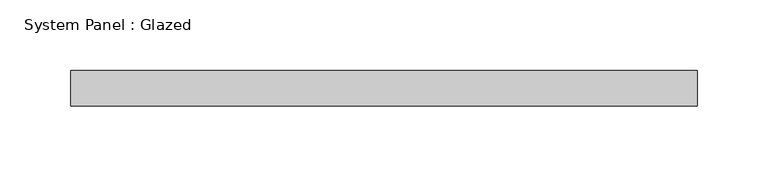
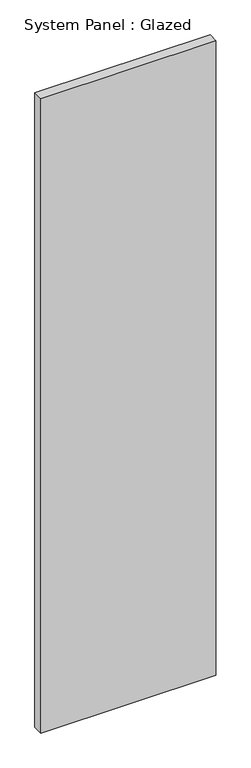
"""IFC4 building model written with IfcOpenShell, lengths in millimetres: plate geometry, System Panel : Glazed."""

from ifc_helpers import new_model, si_unit, origin, origin_with_axes, place, context, project, spatial, polyline, outline, extrude, source, transform, mapped, element, save


def system_panel_glazed_693f0248(model_context):
    return source(origin(), model_context, "Body", "SweptSolid", [
        extrude(outline(polyline([(222.25, 19.05), (-222.25, 19.05), (-222.25, 44.45), (222.25, 44.45), (222.25, 19.05)])), origin_with_axes(), (0.0, 0.0, 1.0), 1701.8),
    ])


if __name__ == "__main__":
    model = new_model("IFC4")
    model_context = context("Model", 3, world=origin())
    ifc_project = project(units=[si_unit("LENGTHUNIT", "METRE", prefix="MILLI")], contexts=[model_context])
    site = spatial("IfcSite", under=ifc_project)
    building = spatial("IfcBuilding", under=site)
    placement = place(None, origin())
    system_panel_glazed_shape = system_panel_glazed_693f0248(model_context)
    element("IfcPlate", 1, ObjectType="System Panel : Glazed", at=placement, inside=building, context=model_context, shape_type="MappedRepresentation", body=[
        mapped(system_panel_glazed_shape, transform((0.0, 0.0, 0.0), x_axis=(1.0, 0.0, 0.0), y_axis=(0.0, 1.0, 0.0), z_axis=(0.0, 0.0, 1.0))),
    ])
    save(model, "model.ifc")

# Revit data of these elements
# Type "System Panel : Glazed"
#   Construction Type Id = "GSP4R"
#   Analytic Construction = "1/8 in Pilkington single glazing"
#   Visual Light Transmittance = 0.9
#   Solar Heat Gain Coefficient = 0.86
#   Heat Transfer Coefficient (U) = 1.18115 BTU/(h·ft²·°F)
#   Define Thermal Properties by = 1
# Element 1 (IfcPlate, "System Panel : Glazed")
#   Materials on its faces: "Glass"
# Materials
#   "Glass": class "Glass", colour RGB 0 128 192, transparency 0.75, Description = "Soda Lime Glass", Cost = 0
